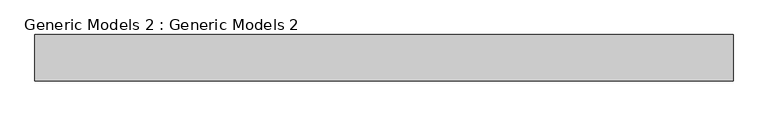
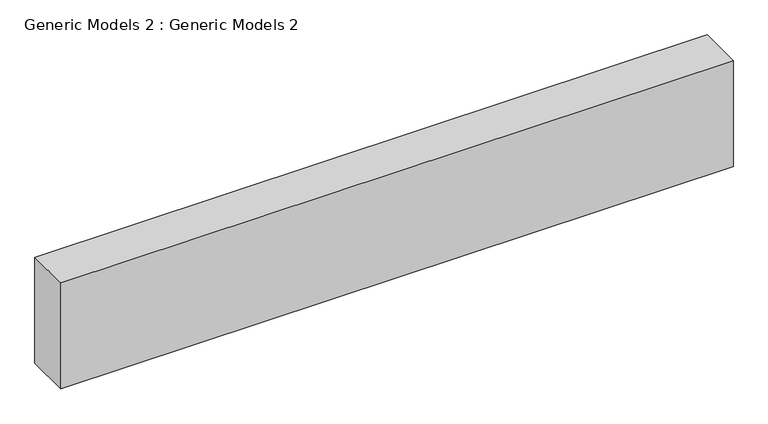
"""IFC4 building model written with IfcOpenShell, lengths in millimetres: proxy geometry, Generic Models 2 : Generic Models 2."""

from ifc_helpers import new_model, si_unit, frame, origin, place, context, project, spatial, polyline, outline, extrude, source, transform, mapped, element, save


def generic_models_2_generic_models_2_5d5211df(model_context):
    return source(origin(), model_context, "Body", "SweptSolid", [
        extrude(outline(polyline([(-4775.3212197, -10871.3980165), (-9347.3212197, -10871.3980165), (-9347.3212197, -10566.5980165), (-4775.3212197, -10566.5980165), (-4775.3212197, -10871.3980165)])), frame((0.0, 0.0, 368.9382078), z_axis=(0.0, 0.0, 1.0), x_axis=(1.0, 0.0, 0.0)), (0.0, 0.0, 1.0), 762.0),
    ])


if __name__ == "__main__":
    model = new_model("IFC4")
    model_context = context("Model", 3, world=origin())
    ifc_project = project(units=[si_unit("LENGTHUNIT", "METRE", prefix="MILLI")], contexts=[model_context])
    site = spatial("IfcSite", under=ifc_project)
    building = spatial("IfcBuilding", under=site)
    placement = place(None, origin())
    generic_models_2_generic_models_2_shape = generic_models_2_generic_models_2_5d5211df(model_context)
    element("IfcBuildingElementProxy", 1, Name="Generic Models 2 : Generic Models 2", ObjectType="Generic Models 2 : Generic Models 2", at=placement, inside=building, context=model_context, shape_type="MappedRepresentation", body=[
        mapped(generic_models_2_generic_models_2_shape, transform((0.0, 0.0, 0.0), x_axis=(1.0, 0.0, 0.0), y_axis=(0.0, 1.0, 0.0), z_axis=(0.0, 0.0, 1.0))),
    ])
    save(model, "model.ifc")

# Revit data of these elements
# Element 1 (IfcBuildingElementProxy, "Generic Models 2 : Generic Models 2")
#   Materials on its faces: "Parking Stripe"
# Materials
#   "Parking Stripe": class "Paint", colour RGB 250 250 91, transparency 0, Cost = 0
